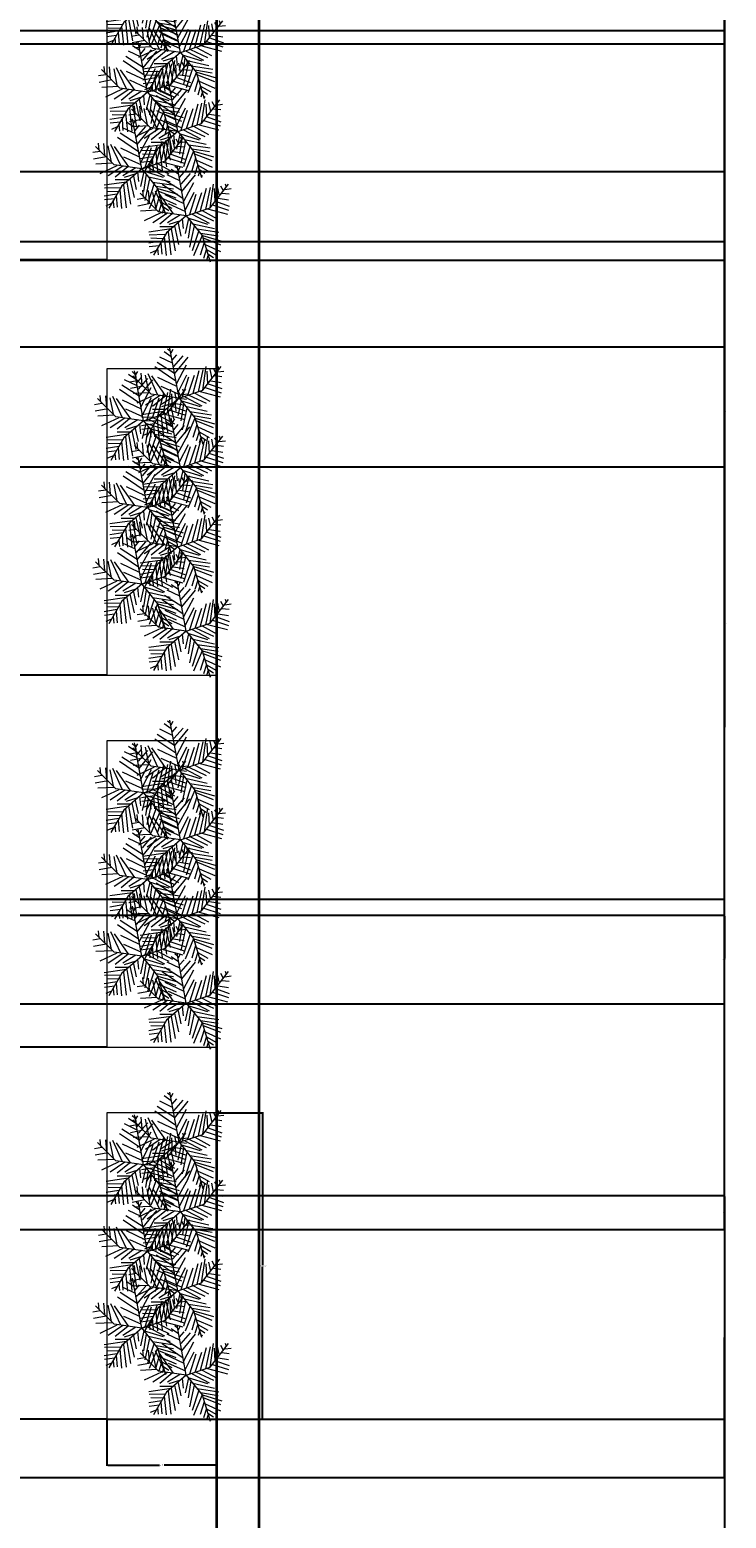
# Model space of a CAD drawing. Units: inches. Extents: x 818 to 1898, y 976 to 2364.
# Tile 47 of 96: x 1750 to 1898, y 1277 to 1594. Entities that reach past the tile are written whole.
import ezdxf

# ---------------------------------------------------------------- set-up
doc = ezdxf.new("R2010")
doc.units = ezdxf.units.IN
doc.header["$LTSCALE"] = 5
doc.header["$MEASUREMENT"] = 0
for name, color, linetype, lineweight in [('A-ANNO-DIMS', 2, 'Continuous', 18), ('C-PROP', 7, 'Continuous', 35), ('L-PLNT-BEDS', 94, 'Continuous', 18)]:
    doc.layers.add(name, color=color, linetype=linetype, lineweight=lineweight)
doc.layers.add('L-PLNT', color=116, linetype='Continuous', lineweight=13, true_color=0x136734)
doc.styles.get("Standard").update_dxf_attribs({"font": 'arial.ttf'})
doc.dimstyles.get("Standard").update_dxf_attribs({"dimtxt": 0.18, "dimasz": 0.18, "dimexe": 0.18, "dimexo": 0.0625, "dimgap": 0.09, "dimtad": 0, "dimtih": 1, "dimtoh": 1, "dimdec": 4, "dimzin": 0, "dimdsep": 46, "dimtxsty": 'Standard', "dimcen": 0.09, "dimadec": 0, "dimazin": 0, "dimtfac": 1, "dimtdec": 4, "dimtofl": 0, "dimtmove": 0, "dimatfit": 3, "dimfxl": 1, "dimtolj": 1, "dimtzin": 0, "dimarcsym": 0})

# ---------------------------------------------------------------- blocks, each defined once
blk = doc.blocks.new('SHRUB-ACCENT')
for p, q in [((8.8, 18.63), (7.25, 19.67)), ((8.53, 19.84), (7.99, 20.28)), ((10.44, 9.82), (8.47, 20.47)), ((8.74, 19.5), (9.21, 20.28)), ((9.01, 17.93), (9.96, 19.06)), ((9.75, 13.42), (5.28, 16.46)), ((9.48, 15.07), (5.82, 17.41)), ((9.08, 17.24), (6.37, 18.54)), ((9.35, 16.54), (11.31, 18.8)), ((9.48, 14.98), (12.39, 18.54)), ((9.89, 12.9), (12.06, 16.89)), ((14.56, 11.16), (15.58, 15.85)), ((15.49, 11.5), (19.41, 16.55)), ((15.51, 11.51), (16.25, 16.54)), ((17, 15.94), (17.41, 14.03)), ((17.68, 16.2), (18.29, 15.16)), ((18.69, 16.63), (18.9, 15.94)), ((1.56, 13.51), (0, 13.25)), ((4.55, 10.66), (0.62, 14.58)), ((1.35, 13.77), (1.22, 15.24)), ((2.3, 15.16), (2.51, 12.72)), ((3.25, 14.72), (3.93, 11.25)), ((3.79, 15.07), (5.89, 10.55)), ((7.72, 10.21), (4.67, 14.55)), ((5.89, 14.29), (9.89, 12.38)), ((10.23, 11.07), (12.12, 14.81)), ((11.17, 10.12), (12.53, 14.37)), ((12.33, 10.47), (13.75, 14.72)), ((13.48, 10.9), (14.76, 15.68)), ((16.39, 15.59), (16.53, 12.9)), ((16.66, 12.9), (19.57, 11.86)), ((17.2, 13.51), (19.44, 13.16)), ((18.02, 14.63), (19.57, 14.46)), ((18.62, 15.42), (19.98, 15.59)), ((2.84, 12.38), (0.14, 11.86)), ((4.2, 10.99), (0.68, 10.81)), ((5.15, 10.47), (1.49, 8.73)), ((6.43, 10.38), (3.32, 8.3)), ((10.44, 9.82), (4.55, 10.66)), ((7.45, 10.21), (4.81, 8.04)), ((10.44, 9.82), (6.23, 6.17)), ((9.21, 10.03), (6.43, 8.3)), ((6.57, 12.38), (10.23, 10.73)), ((10.44, 9.82), (15.49, 11.5)), ((10.44, 9.82), (13.8, 5.61)), ((11.65, 10.12), (15.31, 8.21)), ((12.53, 10.47), (16.19, 8.73)), ((13.82, 10.9), (17, 9.16)), ((14.97, 11.25), (19.17, 10.12)), ((15.98, 12.12), (19.44, 10.99)), ((7.18, 6.99), (2.44, 6.3)), ((7.59, 7.43), (4.81, 7.43)), ((6.57, 6.39), (7.11, 1.52)), ((9.21, 8.73), (6.7, 7.95)), ((7.25, 6.99), (8.06, 2.31)), ((7.92, 7.69), (8.8, 3.69)), ((8.67, 8.21), (9.28, 5.43)), ((9.55, 9.16), (9.75, 7.08)), ((10.9, 9.25), (10.16, 6.04)), ((10.77, 9.34), (14.97, 8.04)), ((11.38, 8.64), (10.84, 5)), ((12.12, 7.69), (11.11, 3.09)), ((13.07, 6.65), (11.65, 2.31)), ((11.85, 8.12), (16.46, 7.08)), ((12.73, 6.99), (17.34, 6.3)), ((5.15, 4.39), (2.44, 3.95)), ((5.89, 5.78), (2.51, 5.69)), ((4.67, 3.43), (2.51, 3.17)), ((5.42, 4.91), (2.91, 5)), ((6.23, 6.17), (3.43, 1.4)), ((5.01, 4.04), (5.21, 1.61)), ((5.76, 5.34), (6.16, 1.35)), ((13.82, 5.6), (11.99, 1.26)), ((14.22, 4.13), (13.41, 1.44)), ((13.48, 6.13), (17.2, 5.52)), ((13.8, 5.61), (15.49, 0)), ((13.88, 5.6), (18.02, 4.39)), ((14.02, 5.08), (17.68, 3.61)), ((14.43, 3.69), (17.74, 2.22)), ((4, 2.39), (2.78, 1.87)), ((4.33, 2.91), (4.47, 1.52)), ((14.7, 2.74), (14.09, 0.74)), ((14.7, 2.65), (16.86, 1.44)), ((15.04, 1.26), (14.76, 0.31)), ((15.04, 1.7), (16.19, 0.92)), ((15.44, 0.48), (15.71, 0.31))]:
    blk.add_line(p, q)
blk = doc.blocks.new('PLANTER-RECT')
at = {"ltscale": 5}
blk.add_lwpolyline([(23.37, 65.17), (0, 65.17), (0, 0), (23.37, 0)], close=True, dxfattribs=at)
blk = doc.blocks.new('*D30')
at = {"layer": 'A-ANNO-DIMS', "color": 0, "lineweight": -2, "ltscale": 5, "transparency": 16777216}
for p, q in [((1789.78, 1363.67), (1799.67, 1363.67)), ((1799.49, 1363.49), (1799.49, 1331.27)), ((1799.49, 1298.68), (1799.49, 1330.9)), ((1789.78, 1298.5), (1799.67, 1298.5))]:
    blk.add_line(p, q, dxfattribs=at)
at = {"layer": 'A-ANNO-DIMS', "color": 0, "ltscale": 5, "transparency": 16777216}
for points in [[(1799.46, 1363.49), (1799.52, 1363.49), (1799.49, 1363.67)], [(1799.46, 1298.68), (1799.52, 1298.68), (1799.49, 1298.5)]]:
    blk.add_solid(points, dxfattribs=at)
at = {"layer": 'Defpoints', "color": 0, "ltscale": 5, "transparency": 16777216}
for p in [(1789.72, 1363.67), (1799.49, 1363.67), (1789.72, 1298.5)]:
    blk.add_point(p, dxfattribs=at)
at = {"layer": 'A-ANNO-DIMS', "color": 0, "ltscale": 5, "transparency": 16777216, "insert": (1799.49, 1331.09), "char_height": 0.18, "attachment_point": 5}
blk.add_mtext('\\A1;PLANTER 65 TYP.', dxfattribs=at)
blk = doc.blocks.new('*D31')
at = {"layer": 'A-ANNO-DIMS', "color": 0, "lineweight": -2, "ltscale": 5, "transparency": 16777216}
for p, q in [((1766.35, 1298.44), (1766.35, 1288.55)), ((1789.72, 1298.44), (1789.72, 1288.55)), ((1766.53, 1288.73), (1777.51, 1288.73)), ((1789.54, 1288.73), (1778.56, 1288.73))]:
    blk.add_line(p, q, dxfattribs=at)
at = {"layer": 'A-ANNO-DIMS', "color": 0, "ltscale": 5, "transparency": 16777216}
for points in [[(1766.53, 1288.76), (1766.53, 1288.7), (1766.35, 1288.73)], [(1789.54, 1288.76), (1789.54, 1288.7), (1789.72, 1288.73)]]:
    blk.add_solid(points, dxfattribs=at)
at = {"layer": 'Defpoints', "color": 0, "ltscale": 5, "transparency": 16777216}
for p in [(1766.35, 1298.5), (1789.72, 1298.5), (1789.72, 1288.73)]:
    blk.add_point(p, dxfattribs=at)
at = {"layer": 'A-ANNO-DIMS', "color": 0, "ltscale": 5, "transparency": 16777216, "insert": (1778.03, 1288.73), "char_height": 0.18, "attachment_point": 5}
blk.add_mtext('\\A1;23 TYP.', dxfattribs=at)
blk = doc.blocks.new('*D66')
at = {"layer": 'A-ANNO-DIMS', "color": 0, "lineweight": -2, "ltscale": 5, "transparency": 16777216}
for p, q in [((1714.73, 1346.02), (1714.73, 975.66)), ((1789.72, 1298.44), (1789.72, 975.66)), ((1714.91, 975.84), (1751.83, 975.84)), ((1789.54, 975.84), (1752.61, 975.84))]:
    blk.add_line(p, q, dxfattribs=at)
at = {"layer": 'A-ANNO-DIMS', "color": 0, "ltscale": 5, "transparency": 16777216}
for points in [[(1714.91, 975.87), (1714.91, 975.81), (1714.73, 975.84)], [(1789.54, 975.87), (1789.54, 975.81), (1789.72, 975.84)]]:
    blk.add_solid(points, dxfattribs=at)
at = {"layer": 'Defpoints', "color": 0, "ltscale": 5, "transparency": 16777216}
for p in [(1714.73, 1346.08), (1789.72, 1298.5), (1789.72, 975.84)]:
    blk.add_point(p, dxfattribs=at)
at = {"layer": 'A-ANNO-DIMS', "color": 0, "ltscale": 5, "transparency": 16777216, "insert": (1752.22, 975.84), "char_height": 0.18, "attachment_point": 5}
blk.add_mtext('\\A1;74.99', dxfattribs=at)
blk = doc.blocks.new('*D70')
at = {"layer": 'A-ANNO-DIMS', "color": 0, "lineweight": -2, "ltscale": 5, "transparency": 16777216}
for p, q in [((1714.79, 1346.08), (1897.92, 1346.08)), ((1897.74, 1345.9), (1897.74, 1274.7)), ((1897.74, 1203.14), (1897.74, 1274.34)), ((1798.78, 1202.96), (1897.92, 1202.96))]:
    blk.add_line(p, q, dxfattribs=at)
at = {"layer": 'A-ANNO-DIMS', "color": 0, "ltscale": 5, "transparency": 16777216}
for points in [[(1897.71, 1345.9), (1897.77, 1345.9), (1897.74, 1346.08)], [(1897.71, 1203.14), (1897.77, 1203.14), (1897.74, 1202.96)]]:
    blk.add_solid(points, dxfattribs=at)
at = {"layer": 'Defpoints', "color": 0, "ltscale": 5, "transparency": 16777216}
for p in [(1714.73, 1346.08), (1897.74, 1346.08), (1798.72, 1202.96)]:
    blk.add_point(p, dxfattribs=at)
at = {"layer": 'A-ANNO-DIMS', "color": 0, "ltscale": 5, "transparency": 16777216, "insert": (1897.74, 1274.52), "char_height": 0.18, "attachment_point": 5}
blk.add_mtext('\\A1;143.1', dxfattribs=at)
blk = doc.blocks.new('*D71')
at = {"layer": 'A-ANNO-DIMS', "color": 0, "lineweight": -2, "ltscale": 5, "transparency": 16777216}
for p, q in [((1714.79, 2053.08), (1897.92, 2053.08)), ((1897.74, 2052.9), (1897.74, 1699.76)), ((1897.74, 1346.26), (1897.74, 1699.4)), ((1714.79, 1346.08), (1897.92, 1346.08))]:
    blk.add_line(p, q, dxfattribs=at)
at = {"layer": 'A-ANNO-DIMS', "color": 0, "ltscale": 5, "transparency": 16777216}
for points in [[(1897.71, 2052.9), (1897.77, 2052.9), (1897.74, 2053.08)], [(1897.71, 1346.26), (1897.77, 1346.26), (1897.74, 1346.08)]]:
    blk.add_solid(points, dxfattribs=at)
at = {"layer": 'Defpoints', "color": 0, "ltscale": 5, "transparency": 16777216}
for p in [(1714.73, 2053.08), (1897.74, 2053.08), (1714.73, 1346.08)]:
    blk.add_point(p, dxfattribs=at)
at = {"layer": 'A-ANNO-DIMS', "color": 0, "ltscale": 5, "transparency": 16777216, "insert": (1897.74, 1699.58), "char_height": 0.18, "attachment_point": 5}
blk.add_mtext('\\A1;707', dxfattribs=at)
blk = doc.blocks.new('*D112')
at = {"layer": 'A-ANNO-DIMS', "color": 0, "lineweight": -2, "ltscale": 5, "transparency": 16777216}
for p, q in [((1135.27, 1405.71), (1897.92, 1405.71)), ((1897.74, 1405.53), (1897.74, 1396.48)), ((1897.74, 1387.07), (1897.74, 1396.12)), ((1135.27, 1386.89), (1897.92, 1386.89))]:
    blk.add_line(p, q, dxfattribs=at)
at = {"layer": 'A-ANNO-DIMS', "color": 0, "ltscale": 5, "transparency": 16777216}
for points in [[(1897.71, 1405.53), (1897.77, 1405.53), (1897.74, 1405.71)], [(1897.71, 1387.07), (1897.77, 1387.07), (1897.74, 1386.89)]]:
    blk.add_solid(points, dxfattribs=at)
at = {"layer": 'Defpoints', "color": 0, "ltscale": 5, "transparency": 16777216}
for p in [(1135.21, 1405.71), (1135.21, 1386.89), (1897.74, 1386.89)]:
    blk.add_point(p, dxfattribs=at)
at = {"layer": 'A-ANNO-DIMS', "color": 0, "ltscale": 5, "transparency": 16777216, "insert": (1897.74, 1396.3), "char_height": 0.18, "attachment_point": 5}
blk.add_mtext('\\A1;18.824', dxfattribs=at)
blk = doc.blocks.new('*D113')
at = {"layer": 'A-ANNO-DIMS', "color": 0, "lineweight": -2, "ltscale": 5, "transparency": 16777216}
for p, q in [((1430.79, 1346.08), (1897.92, 1346.08)), ((1897.74, 1345.9), (1897.74, 1316.26)), ((1897.74, 1286.26), (1897.74, 1315.9)), ((1430.79, 1286.08), (1897.92, 1286.08))]:
    blk.add_line(p, q, dxfattribs=at)
at = {"layer": 'A-ANNO-DIMS', "color": 0, "ltscale": 5, "transparency": 16777216}
for points in [[(1897.71, 1345.9), (1897.77, 1345.9), (1897.74, 1346.08)], [(1897.71, 1286.26), (1897.77, 1286.26), (1897.74, 1286.08)]]:
    blk.add_solid(points, dxfattribs=at)
at = {"layer": 'Defpoints', "color": 0, "ltscale": 5, "transparency": 16777216}
for p in [(1430.73, 1346.08), (1897.74, 1346.08), (1430.73, 1286.08)]:
    blk.add_point(p, dxfattribs=at)
at = {"layer": 'A-ANNO-DIMS', "color": 0, "ltscale": 5, "transparency": 16777216, "insert": (1897.74, 1316.08), "char_height": 0.18, "attachment_point": 5}
blk.add_mtext('\\A1;60', dxfattribs=at)
blk = doc.blocks.new('*D114')
at = {"layer": 'A-ANNO-DIMS', "color": 0, "lineweight": -2, "ltscale": 5, "transparency": 16777216}
for p, q in [((1766.41, 1298.5), (1897.92, 1298.5)), ((1897.74, 1298.32), (1897.74, 1250.92)), ((1897.74, 1203.14), (1897.74, 1250.55)), ((1798.78, 1202.96), (1897.92, 1202.96))]:
    blk.add_line(p, q, dxfattribs=at)
at = {"layer": 'A-ANNO-DIMS', "color": 0, "ltscale": 5, "transparency": 16777216}
for points in [[(1897.71, 1298.32), (1897.77, 1298.32), (1897.74, 1298.5)], [(1897.71, 1203.14), (1897.77, 1203.14), (1897.74, 1202.96)]]:
    blk.add_solid(points, dxfattribs=at)
at = {"layer": 'Defpoints', "color": 0, "ltscale": 5, "transparency": 16777216}
for p in [(1766.35, 1298.5), (1897.74, 1298.5), (1798.72, 1202.96)]:
    blk.add_point(p, dxfattribs=at)
at = {"layer": 'A-ANNO-DIMS', "color": 0, "ltscale": 5, "transparency": 16777216, "insert": (1897.74, 1250.73), "char_height": 0.18, "attachment_point": 5}
blk.add_mtext('\\A1;95.54', dxfattribs=at)
blk = doc.blocks.new('*D115')
at = {"layer": 'A-ANNO-DIMS', "color": 0, "lineweight": -2, "ltscale": 5, "transparency": 16777216}
for p, q in [((1766.29, 1377.66), (818.03, 1377.66)), ((818.21, 1377.48), (818.21, 1338.26)), ((818.21, 1298.68), (818.21, 1337.9)), ((1766.29, 1298.5), (818.03, 1298.5))]:
    blk.add_line(p, q, dxfattribs=at)
at = {"layer": 'A-ANNO-DIMS', "color": 0, "ltscale": 5, "transparency": 16777216}
for points in [[(818.18, 1377.48), (818.24, 1377.48), (818.21, 1377.66)], [(818.18, 1298.68), (818.24, 1298.68), (818.21, 1298.5)]]:
    blk.add_solid(points, dxfattribs=at)
at = {"layer": 'Defpoints', "color": 0, "ltscale": 5, "transparency": 16777216}
for p in [(818.21, 1377.66), (1766.35, 1377.66), (1766.35, 1298.5)]:
    blk.add_point(p, dxfattribs=at)
at = {"layer": 'A-ANNO-DIMS', "color": 0, "ltscale": 5, "transparency": 16777216, "insert": (818.21, 1338.08), "char_height": 0.18, "attachment_point": 5}
blk.add_mtext('\\A1;79.15', dxfattribs=at)
blk = doc.blocks.new('*D116')
at = {"layer": 'A-ANNO-DIMS', "color": 0, "lineweight": -2, "ltscale": 5, "transparency": 16777216}
for p, q in [((1766.29, 1456.81), (818.03, 1456.81)), ((818.21, 1456.63), (818.21, 1417.41)), ((818.21, 1377.84), (818.21, 1417.05)), ((1766.29, 1377.66), (818.03, 1377.66))]:
    blk.add_line(p, q, dxfattribs=at)
at = {"layer": 'A-ANNO-DIMS', "color": 0, "ltscale": 5, "transparency": 16777216}
for points in [[(818.18, 1456.63), (818.24, 1456.63), (818.21, 1456.81)], [(818.18, 1377.84), (818.24, 1377.84), (818.21, 1377.66)]]:
    blk.add_solid(points, dxfattribs=at)
at = {"layer": 'Defpoints', "color": 0, "ltscale": 5, "transparency": 16777216}
for p in [(818.21, 1456.81), (1766.35, 1456.81), (1766.35, 1377.66)]:
    blk.add_point(p, dxfattribs=at)
at = {"layer": 'A-ANNO-DIMS', "color": 0, "ltscale": 5, "transparency": 16777216, "insert": (818.21, 1417.23), "char_height": 0.18, "attachment_point": 5}
blk.add_mtext('\\A1;79.15', dxfattribs=at)
blk = doc.blocks.new('*D117')
at = {"layer": 'A-ANNO-DIMS', "color": 0, "lineweight": -2, "ltscale": 5, "transparency": 16777216}
for p, q in [((1766.29, 1545.18), (818.03, 1545.18)), ((818.21, 1545), (818.21, 1501.18)), ((818.21, 1456.99), (818.21, 1500.81)), ((1766.29, 1456.81), (818.03, 1456.81))]:
    blk.add_line(p, q, dxfattribs=at)
at = {"layer": 'A-ANNO-DIMS', "color": 0, "ltscale": 5, "transparency": 16777216}
for points in [[(818.18, 1545), (818.24, 1545), (818.21, 1545.18)], [(818.18, 1456.99), (818.24, 1456.99), (818.21, 1456.81)]]:
    blk.add_solid(points, dxfattribs=at)
at = {"layer": 'Defpoints', "color": 0, "ltscale": 5, "transparency": 16777216}
for p in [(818.21, 1545.18), (1766.35, 1545.18), (1766.35, 1456.81)]:
    blk.add_point(p, dxfattribs=at)
at = {"layer": 'A-ANNO-DIMS', "color": 0, "ltscale": 5, "transparency": 16777216, "insert": (818.21, 1501), "char_height": 0.18, "attachment_point": 5}
blk.add_mtext('\\A1;88.37', dxfattribs=at)
blk = doc.blocks.new('*D118')
at = {"layer": 'A-ANNO-DIMS', "color": 0, "lineweight": -2, "ltscale": 5, "transparency": 16777216}
for p, q in [((1766.29, 1627.51), (818.03, 1627.51)), ((818.21, 1627.33), (818.21, 1586.53)), ((818.21, 1545.36), (818.21, 1586.16)), ((1766.29, 1545.18), (818.03, 1545.18))]:
    blk.add_line(p, q, dxfattribs=at)
at = {"layer": 'A-ANNO-DIMS', "color": 0, "ltscale": 5, "transparency": 16777216}
for points in [[(818.18, 1627.33), (818.24, 1627.33), (818.21, 1627.51)], [(818.18, 1545.36), (818.24, 1545.36), (818.21, 1545.18)]]:
    blk.add_solid(points, dxfattribs=at)
at = {"layer": 'Defpoints', "color": 0, "ltscale": 5, "transparency": 16777216}
for p in [(818.21, 1627.51), (1766.35, 1627.51), (1766.35, 1545.18)]:
    blk.add_point(p, dxfattribs=at)
at = {"layer": 'A-ANNO-DIMS', "color": 0, "ltscale": 5, "transparency": 16777216, "insert": (818.21, 1586.34), "char_height": 0.18, "attachment_point": 5}
blk.add_mtext('\\A1;82.32', dxfattribs=at)
blk = doc.blocks.new('*D170')
at = {"layer": 'A-ANNO-DIMS', "color": 0, "lineweight": -2, "ltscale": 5, "transparency": 16777216}
for p, q in [((1430.79, 1600.08), (1897.92, 1600.08)), ((1897.74, 1599.9), (1897.74, 1550.76)), ((1897.74, 1501.26), (1897.74, 1550.4)), ((1430.79, 1501.08), (1897.92, 1501.08))]:
    blk.add_line(p, q, dxfattribs=at)
at = {"layer": 'A-ANNO-DIMS', "color": 0, "ltscale": 5, "transparency": 16777216}
for points in [[(1897.71, 1599.9), (1897.77, 1599.9), (1897.74, 1600.08)], [(1897.71, 1501.26), (1897.77, 1501.26), (1897.74, 1501.08)]]:
    blk.add_solid(points, dxfattribs=at)
at = {"layer": 'Defpoints', "color": 0, "ltscale": 5, "transparency": 16777216}
for p in [(1430.73, 1600.08), (1897.74, 1600.08), (1430.73, 1501.08)]:
    blk.add_point(p, dxfattribs=at)
at = {"layer": 'A-ANNO-DIMS', "color": 0, "ltscale": 5, "transparency": 16777216, "insert": (1897.74, 1550.58), "char_height": 0.18, "attachment_point": 5}
blk.add_mtext('\\A1;99', dxfattribs=at)
blk = doc.blocks.new('*D184')
at = {"layer": 'A-ANNO-DIMS', "color": 0, "lineweight": -2, "ltscale": 5, "transparency": 16777216}
for p, q in [((1737.9, 1593.92), (1897.92, 1593.92)), ((1897.74, 1593.74), (1897.74, 1571.68)), ((1897.74, 1549.26), (1897.74, 1571.32)), ((1737.9, 1549.08), (1897.92, 1549.08))]:
    blk.add_line(p, q, dxfattribs=at)
at = {"layer": 'A-ANNO-DIMS', "color": 0, "ltscale": 5, "transparency": 16777216}
for points in [[(1897.71, 1593.74), (1897.77, 1593.74), (1897.74, 1593.92)], [(1897.71, 1549.26), (1897.77, 1549.26), (1897.74, 1549.08)]]:
    blk.add_solid(points, dxfattribs=at)
at = {"layer": 'Defpoints', "color": 0, "ltscale": 5, "transparency": 16777216}
for p in [(1737.84, 1593.92), (1897.74, 1593.92), (1737.84, 1549.08)]:
    blk.add_point(p, dxfattribs=at)
at = {"layer": 'A-ANNO-DIMS', "color": 0, "ltscale": 5, "transparency": 16777216, "insert": (1897.74, 1571.5), "char_height": 0.18, "attachment_point": 5}
blk.add_mtext('\\A1;44.84', dxfattribs=at)
blk = doc.blocks.new('*D188')
at = {"layer": 'A-ANNO-DIMS', "color": 0, "lineweight": -2, "ltscale": 5, "transparency": 16777216}
for p, q in [((1714.79, 1545.08), (1897.92, 1545.08)), ((1897.74, 1544.9), (1897.74, 1445.76)), ((1897.74, 1346.26), (1897.74, 1445.4)), ((1714.79, 1346.08), (1897.92, 1346.08))]:
    blk.add_line(p, q, dxfattribs=at)
at = {"layer": 'A-ANNO-DIMS', "color": 0, "ltscale": 5, "transparency": 16777216}
for points in [[(1897.71, 1544.9), (1897.77, 1544.9), (1897.74, 1545.08)], [(1897.71, 1346.26), (1897.77, 1346.26), (1897.74, 1346.08)]]:
    blk.add_solid(points, dxfattribs=at)
at = {"layer": 'Defpoints', "color": 0, "ltscale": 5, "transparency": 16777216}
for p in [(1714.73, 1545.08), (1897.74, 1545.08), (1714.73, 1346.08)]:
    blk.add_point(p, dxfattribs=at)
at = {"layer": 'A-ANNO-DIMS', "color": 0, "ltscale": 5, "transparency": 16777216, "insert": (1897.74, 1445.58), "char_height": 0.18, "attachment_point": 5}
blk.add_mtext('\\A1;199', dxfattribs=at)
blk = doc.blocks.new('*D193')
at = {"layer": 'A-ANNO-DIMS', "color": 0, "lineweight": -2, "ltscale": 5, "transparency": 16777216}
for p, q in [((1660.38, 1346.08), (1897.92, 1346.08)), ((1897.74, 1345.9), (1897.74, 1342.65)), ((1897.74, 1339.05), (1897.74, 1342.29)), ((1660.38, 1338.87), (1897.92, 1338.87))]:
    blk.add_line(p, q, dxfattribs=at)
at = {"layer": 'A-ANNO-DIMS', "color": 0, "ltscale": 5, "transparency": 16777216}
for points in [[(1897.71, 1345.9), (1897.77, 1345.9), (1897.74, 1346.08)], [(1897.71, 1339.05), (1897.77, 1339.05), (1897.74, 1338.87)]]:
    blk.add_solid(points, dxfattribs=at)
at = {"layer": 'Defpoints', "color": 0, "ltscale": 5, "transparency": 16777216}
for p in [(1660.31, 1346.08), (1897.74, 1346.08), (1660.31, 1338.87)]:
    blk.add_point(p, dxfattribs=at)
at = {"layer": 'A-ANNO-DIMS', "color": 0, "ltscale": 5, "transparency": 16777216, "insert": (1897.74, 1342.47), "char_height": 0.18, "attachment_point": 5}
blk.add_mtext('\\A1;7.213', dxfattribs=at)
blk = doc.blocks.new('*D197')
at = {"layer": 'A-ANNO-DIMS', "color": 0, "lineweight": -2, "ltscale": 5, "transparency": 16777216}
for p, q in [((1457.79, 1526.67), (1897.92, 1526.67)), ((1897.74, 1526.49), (1897.74, 1468.08)), ((1897.74, 1409.3), (1897.74, 1467.71)), ((1457.79, 1409.12), (1897.92, 1409.12))]:
    blk.add_line(p, q, dxfattribs=at)
at = {"layer": 'A-ANNO-DIMS', "color": 0, "ltscale": 5, "transparency": 16777216}
for points in [[(1897.71, 1526.49), (1897.77, 1526.49), (1897.74, 1526.67)], [(1897.71, 1409.3), (1897.77, 1409.3), (1897.74, 1409.12)]]:
    blk.add_solid(points, dxfattribs=at)
at = {"layer": 'Defpoints', "color": 0, "ltscale": 5, "transparency": 16777216}
for p in [(1457.73, 1526.67), (1897.74, 1526.67), (1457.73, 1409.12)]:
    blk.add_point(p, dxfattribs=at)
at = {"layer": 'A-ANNO-DIMS', "color": 0, "ltscale": 5, "transparency": 16777216, "insert": (1897.74, 1467.89), "char_height": 0.18, "attachment_point": 5}
blk.add_mtext('\\A1;117.55', dxfattribs=at)
blk = doc.blocks.new('*D199')
at = {"layer": 'A-ANNO-DIMS', "color": 0, "lineweight": -2, "ltscale": 5, "transparency": 16777216}
for p, q in [((1559.79, 1687.08), (1897.92, 1687.08)), ((1897.74, 1686.9), (1897.74, 1513.15)), ((1897.74, 1339.05), (1897.74, 1512.79)), ((1660.38, 1338.87), (1897.92, 1338.87))]:
    blk.add_line(p, q, dxfattribs=at)
at = {"layer": 'A-ANNO-DIMS', "color": 0, "ltscale": 5, "transparency": 16777216}
for points in [[(1897.71, 1686.9), (1897.77, 1686.9), (1897.74, 1687.08)], [(1897.71, 1339.05), (1897.77, 1339.05), (1897.74, 1338.87)]]:
    blk.add_solid(points, dxfattribs=at)
at = {"layer": 'Defpoints', "color": 0, "ltscale": 5, "transparency": 16777216}
for p in [(1559.73, 1687.08), (1897.74, 1687.08), (1660.31, 1338.87)]:
    blk.add_point(p, dxfattribs=at)
at = {"layer": 'A-ANNO-DIMS', "color": 0, "ltscale": 5, "transparency": 16777216, "insert": (1897.74, 1512.97), "char_height": 0.18, "attachment_point": 5}
blk.add_mtext('\\A1;348.2', dxfattribs=at)
blk = doc.blocks.new('*D202')
at = {"layer": 'A-ANNO-DIMS', "color": 0, "lineweight": -2, "ltscale": 5, "transparency": 16777216}
for p, q in [((1705.79, 1591.08), (1897.92, 1591.08)), ((1897.74, 1590.9), (1897.74, 1577.7)), ((1897.74, 1564.15), (1897.74, 1577.34)), ((1704.79, 1563.97), (1897.92, 1563.97))]:
    blk.add_line(p, q, dxfattribs=at)
at = {"layer": 'A-ANNO-DIMS', "color": 0, "ltscale": 5, "transparency": 16777216}
for points in [[(1897.71, 1590.9), (1897.77, 1590.9), (1897.74, 1591.08)], [(1897.71, 1564.15), (1897.77, 1564.15), (1897.74, 1563.97)]]:
    blk.add_solid(points, dxfattribs=at)
at = {"layer": 'Defpoints', "color": 0, "ltscale": 5, "transparency": 16777216}
for p in [(1705.73, 1591.08), (1897.74, 1591.08), (1704.73, 1563.97)]:
    blk.add_point(p, dxfattribs=at)
at = {"layer": 'A-ANNO-DIMS', "color": 0, "ltscale": 5, "transparency": 16777216, "insert": (1897.74, 1577.52), "char_height": 0.18, "attachment_point": 5}
blk.add_mtext('\\A1;27.11', dxfattribs=at)

msp = doc.modelspace()

# ---------------------------------------------------------------- linework, layer by layer
at = {"layer": 'C-PROP', "ltscale": 5}
for p, q in [((1798.7173, 1202.9642), (1798.7173, 2294.2171)), ((1789.7173, 1211.9642), (1789.7173, 2285.2171))]:
    msp.add_line(p, q, dxfattribs=at)

# ---------------------------------------------------------------- block references
at = {"layer": 'L-PLNT'}
for p in [(1763.7314, 1589.4538), (1771.5761, 1579.4457), (1764.5652, 1571.0326), (1770.9913, 1562.6539), (1763.3302, 1554.7093), (1772.8128, 1544.7235), (1771.257, 1505.8987), (1763.7314, 1501.0798), (1771.5761, 1491.0718), (1764.5652, 1482.6587), (1770.9913, 1474.28), (1763.3302, 1466.3354), (1772.8128, 1456.3495), (1771.257, 1426.7464), (1763.7314, 1421.9275), (1771.5761, 1411.9194), (1764.5652, 1403.5063), (1770.9913, 1395.1277), (1763.3302, 1387.1831), (1772.8128, 1377.1972), (1771.257, 1347.594), (1763.7314, 1342.7752), (1771.5761, 1332.7671), (1764.5652, 1324.354), (1770.9913, 1315.9753), (1763.3302, 1308.0308), (1772.8128, 1298.0449)]:
    msp.add_blockref('SHRUB-ACCENT', p, dxfattribs=at)
at = {"layer": 'L-PLNT-BEDS'}
for p in [(1766.352, 1545.1826), (1766.352, 1545.1826), (1766.352, 1456.8087), (1766.352, 1456.8087), (1766.352, 1377.6564), (1766.352, 1377.6564), (1766.352, 1298.504), (1766.352, 1298.504)]:
    msp.add_blockref('PLANTER-RECT', p, dxfattribs=at)

# ---------------------------------------------------------------- dimensions: what is measured, and where the dimension line sits
at = {"layer": 'A-ANNO-DIMS', "ltscale": 5}
for base, p1, p2, override, picture, middle in [((1897.736, 2053.0782), (1714.7251, 1346.0782), (1714.7251, 2053.0782), {"dimdec": 0, "dimlfac": 1, "dimrnd": 0, "dimzin": 0, "dimdsep": 46, "dimlunit": 2}, '*D71', (1897.736, 1699.5782)), ((1897.736, 1687.0782), (1660.3141, 1338.8654), (1559.7251, 1687.0782), {"dimdec": 1, "dimlfac": 1, "dimrnd": 0, "dimzin": 0, "dimdsep": 46, "dimlunit": 2}, '*D199', (1897.736, 1512.9718)), ((818.2059, 1627.5052), (1766.3524, 1545.1827), (1766.3524, 1627.5052), {"dimdec": 2, "dimlfac": 1, "dimrnd": 0, "dimzin": 0, "dimdsep": 46, "dimlunit": 2}, '*D118', (818.2059, 1586.3439)), ((1897.736, 1600.0782), (1430.7251, 1501.0782), (1430.7251, 1600.0782), {"dimdec": 0, "dimlfac": 1, "dimrnd": 0, "dimzin": 0, "dimdsep": 46, "dimlunit": 2}, '*D170', (1897.736, 1550.5782)), ((1897.736, 1593.9175), (1737.8409, 1549.0782), (1737.8409, 1593.9175), {"dimdec": 2, "dimlfac": 1, "dimrnd": 0, "dimzin": 0, "dimdsep": 46, "dimlunit": 2}, '*D184', (1897.736, 1571.4979)), ((1897.736, 1591.0782), (1704.7251, 1563.9657), (1705.7251, 1591.0782), {"dimdec": 2, "dimlfac": 1, "dimrnd": 0, "dimzin": 0, "dimdsep": 46, "dimlunit": 2}, '*D202', (1897.736, 1577.522)), ((818.2059, 1545.1827), (1766.3524, 1456.8088), (1766.3524, 1545.1827), {"dimdec": 2, "dimlfac": 1, "dimrnd": 0, "dimzin": 0, "dimdsep": 46, "dimlunit": 2}, '*D117', (818.2059, 1500.9957)), ((1897.736, 1545.0782), (1714.7251, 1346.0782), (1714.7251, 1545.0782), {"dimdec": 0, "dimlfac": 1, "dimrnd": 0, "dimzin": 0, "dimdsep": 46, "dimlunit": 2}, '*D188', (1897.736, 1445.5782)), ((1897.736, 1526.6712), (1457.7251, 1409.1177), (1457.7251, 1526.6712), {"dimdec": 2, "dimlfac": 1, "dimrnd": 0, "dimzin": 0, "dimdsep": 46, "dimlunit": 2}, '*D197', (1897.736, 1467.8945)), ((818.2059, 1456.8088), (1766.3524, 1377.6564), (1766.3524, 1456.8088), {"dimdec": 2, "dimlfac": 1, "dimrnd": 0, "dimzin": 0, "dimdsep": 46, "dimlunit": 2}, '*D116', (818.2059, 1417.2326)), ((1897.736, 1386.8851), (1135.2058, 1405.7088), (1135.2058, 1386.8851), {"dimdec": 3, "dimlfac": 1, "dimrnd": 0, "dimzin": 0, "dimdsep": 46, "dimlunit": 2}, '*D112', (1897.736, 1396.297)), ((818.2059, 1377.6564), (1766.3524, 1298.5041), (1766.3524, 1377.6564), {"dimdec": 2, "dimlfac": 1, "dimrnd": 0, "dimzin": 0, "dimdsep": 46, "dimlunit": 2}, '*D115', (818.2059, 1338.0803)), ((1897.736, 1346.0782), (1430.7251, 1286.0782), (1430.7251, 1346.0782), {"dimdec": 0, "dimlfac": 1, "dimrnd": 0, "dimzin": 0, "dimdsep": 46, "dimlunit": 2}, '*D113', (1897.736, 1316.0782)), ((1897.736, 1346.0782), (1660.3141, 1338.8654), (1660.3141, 1346.0782), {"dimdec": 3, "dimlfac": 1, "dimrnd": 0, "dimzin": 0, "dimdsep": 46, "dimlunit": 2}, '*D193', (1897.736, 1342.4718)), ((1897.736, 1346.0782), (1798.7173, 1202.9642), (1714.7251, 1346.0782), {"dimdec": 1, "dimlfac": 1, "dimrnd": 0, "dimzin": 0, "dimdsep": 46, "dimlunit": 2}, '*D70', (1897.736, 1274.5212)), ((1897.736, 1298.5041), (1798.7173, 1202.9642), (1766.3524, 1298.5041), {"dimdec": 2, "dimlfac": 1, "dimrnd": 0, "dimzin": 0, "dimdsep": 46, "dimlunit": 2}, '*D114', (1897.736, 1250.7342))]:
    dim = msp.add_linear_dim(base=base, p1=p1, p2=p2, angle=90, dimstyle='Standard', override=override, dxfattribs=at)
    dim.commit()
    dim.dimension.update_dxf_attribs({"geometry": picture, "text_midpoint": middle})
dim = msp.add_linear_dim(base=(1799.4921, 1363.6693), p1=(1789.7173, 1298.5041), p2=(1789.7173, 1363.6693), angle=90, text='PLANTER <> TYP.', dimstyle='Standard', override={"dimdec": 0, "dimlfac": 1, "dimrnd": 0, "dimzin": 0, "dimdsep": 46, "dimlunit": 2}, dxfattribs=at)
dim.commit()
dim.dimension.update_dxf_attribs({"geometry": '*D30', "text_midpoint": (1799.4921, 1331.0867)})
dim = msp.add_linear_dim(base=(1789.7173, 975.8433), p1=(1714.7251, 1346.0782), p2=(1789.7173, 1298.5041), dimstyle='Standard', override={"dimdec": 2, "dimlfac": 1, "dimrnd": 0, "dimzin": 0, "dimdsep": 46, "dimlunit": 2}, dxfattribs=at)
dim.commit()
dim.dimension.update_dxf_attribs({"geometry": '*D66', "text_midpoint": (1752.2212, 975.8433)})
dim = msp.add_linear_dim(base=(1789.7173, 1288.7293), p1=(1766.3524, 1298.5041), p2=(1789.7173, 1298.5041), text='<> TYP.', dimstyle='Standard', override={"dimdec": 0, "dimlfac": 1, "dimrnd": 0, "dimzin": 0, "dimdsep": 46, "dimlunit": 2}, dxfattribs=at)
dim.commit()
dim.dimension.update_dxf_attribs({"geometry": '*D31', "text_midpoint": (1778.0348, 1288.7293)})

doc.saveas('drawing.dxf')
